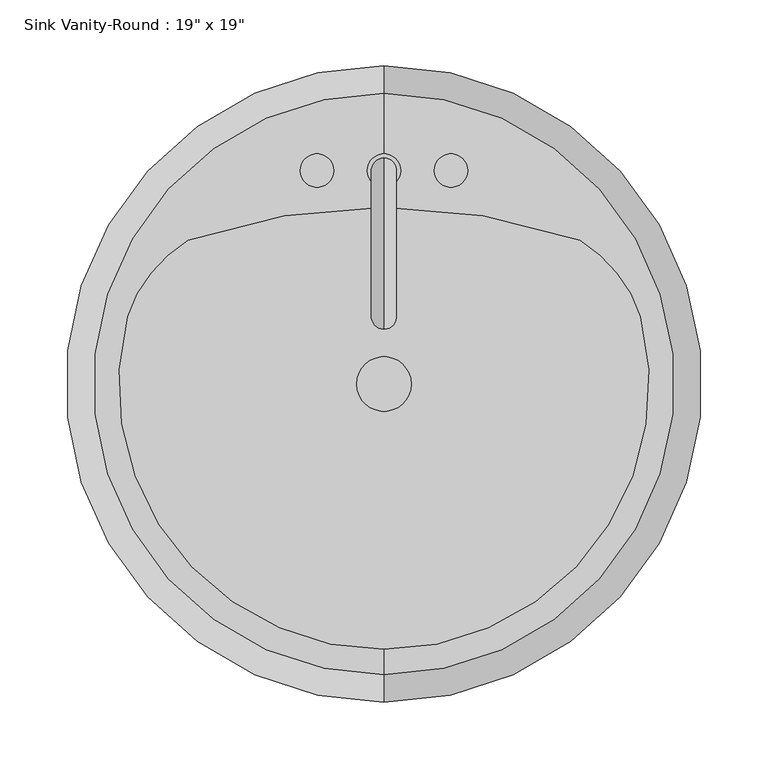
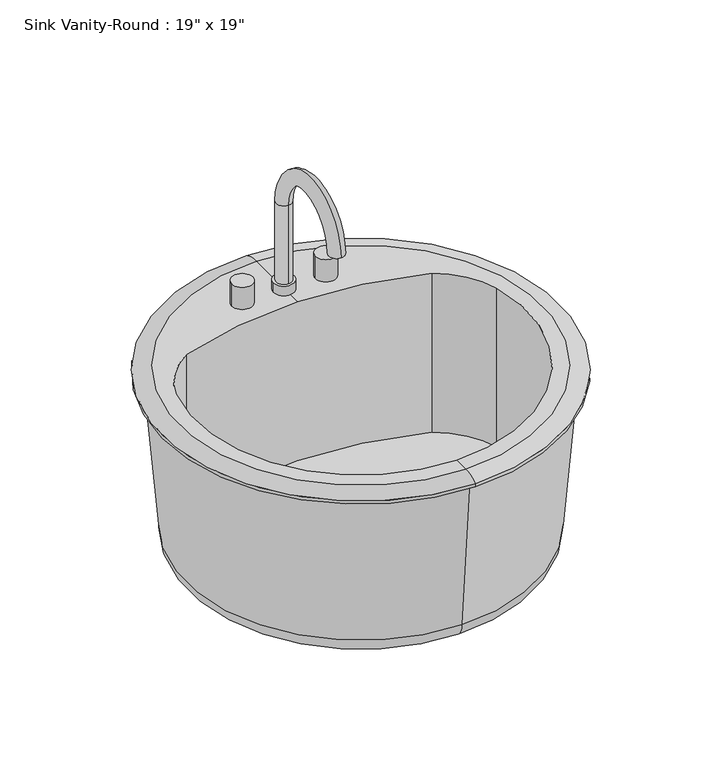
"""IFC4 building model written with IfcOpenShell, lengths in millimetres: flow terminal geometry."""

from ifc_helpers import new_model, si_unit, point, frame, frame_2d, origin, place, context, project, spatial, polyline, circle_curve, ellipse_curve, trimmed, segment, composite_curve, outline, extrude, source, transform, mapped, element, save
from ifc_brep_helpers import plane_surface, cylinder_surface, revolved_surface, advanced_brep


def flow_terminal_d49f872f(model_context):
    return source(origin(), model_context, "Body", "SolidModel", [
        advanced_brep(
        [(83.9517406, 247.0927185, 796.925), (109.3517406, 247.0927185, 796.925), (96.6517406, 237.5677185, 909.6375), (96.6517406, 256.6177185, 909.6375), (96.6517406, 256.6177185, 809.1602909), (96.6517406, 237.5677185, 809.1602909), (96.6517406, 145.7775038, 909.6375), (96.6517406, 126.7275038, 909.6375), (83.9517406, 247.0927185, 809.1602909), (109.3517406, 247.0927185, 809.1602909)],
        [
            (0, 1, circle_curve(frame((96.6517406, 247.0927185, 796.925), z_axis=(0.0, 0.0, -1.0), x_axis=(1.0, 0.0, 0.0)), 12.7)),
            (1, 0, circle_curve(frame((96.6517406, 247.0927185, 796.925), z_axis=(0.0, 0.0, -1.0), x_axis=(1.0, 0.0, 0.0)), 12.7)),
            (2, 3, circle_curve(frame((96.6517406, 247.0927185, 909.6375), z_axis=(0.0, 0.0, -1.0), x_axis=(0.0, 1.0, 0.0)), 9.525)),
            (3, 4),
            (4, 5, circle_curve(frame((96.6517406, 247.0927185, 809.1602909), z_axis=(0.0, 0.0, 1.0), x_axis=(0.0, 1.0, 0.0)), 9.525)),
            (5, 2),
            (3, 2, circle_curve(frame((96.6517406, 247.0927185, 909.6375), z_axis=(0.0, 0.0, -1.0), x_axis=(0.0, 1.0, 0.0)), 9.525)),
            (5, 4, circle_curve(frame((96.6517406, 247.0927185, 809.1602909), z_axis=(0.0, 0.0, 1.0), x_axis=(0.0, 1.0, 0.0)), 9.525)),
            (6, 7, circle_curve(frame((96.6517406, 136.2525038, 909.6375), z_axis=(0.0, 0.0, -1.0), x_axis=(0.0, -1.0, 0.0)), 9.525)),
            (7, 6, circle_curve(frame((96.6517406, 136.2525038, 909.6375), z_axis=(0.0, 0.0, -1.0), x_axis=(0.0, -1.0, 0.0)), 9.525)),
            (2, 6, circle_curve(frame((96.6517406, 191.6726112, 909.6375), z_axis=(1.0, 0.0, 0.0), x_axis=(0.0, 1.0, 0.0)), 45.8951073)),
            (7, 3, circle_curve(frame((96.6517406, 191.6726112, 909.6375), z_axis=(-1.0, 0.0, 0.0), x_axis=(0.0, 1.0, 0.0)), 64.9451073)),
            (8, 9, circle_curve(frame((96.6517406, 247.0927185, 809.1602909), z_axis=(0.0, 0.0, 1.0), x_axis=(1.0, 0.0, 0.0)), 12.7)),
            (9, 8, circle_curve(frame((96.6517406, 247.0927185, 809.1602909), z_axis=(0.0, 0.0, 1.0), x_axis=(1.0, 0.0, 0.0)), 12.7)),
            (8, 0),
            (1, 9),
        ],
        [
            plane_surface(frame((96.6517406, 237.5677185, 796.925), z_axis=(0.0, 0.0, -1.0), x_axis=(1.0, 0.0, 0.0))),
            cylinder_surface(frame((96.6517406, 247.0927185, 796.925), z_axis=(0.0, 0.0, -1.0), x_axis=(0.0, 1.0, 0.0)), 9.525),
            plane_surface(frame((96.6517406, 191.6726112, 909.6375), z_axis=(0.0, 0.0, -1.0), x_axis=(0.0, -1.0, 0.0))),
            revolved_surface(trimmed(ellipse_curve(frame((96.6517406, 247.0927185, 909.6375), z_axis=(0.0, 0.0, -1.0), x_axis=(0.0, 1.0, 0.0)), 9.525, 9.525), [point((96.6517406, 237.5677185, 909.6375))], [point((96.6517406, 256.6177185, 909.6375))], True, "CARTESIAN"), (96.6517406, 191.6726112, 909.6375), (1.0, 0.0, 0.0)),
            revolved_surface(trimmed(ellipse_curve(frame((96.6517406, 247.0927185, 909.6375), z_axis=(0.0, 0.0, -1.0), x_axis=(0.0, 1.0, 0.0)), 9.525, 9.525), [point((96.6517406, 256.6177185, 909.6375))], [point((96.6517406, 237.5677185, 909.6375))], True, "CARTESIAN"), (96.6517406, 191.6726112, 909.6375), (1.0, 0.0, 0.0)),
            plane_surface(frame((109.3517406, 247.0927185, 809.1602909), z_axis=(0.0, 0.0, 1.0), x_axis=(0.0, 1.0, 0.0))),
            cylinder_surface(frame((96.6517406, 247.0927185, 796.925), z_axis=(0.0, 0.0, 1.0), x_axis=(1.0, 0.0, 0.0)), 12.7),
        ],
        [
            (0, [[1, 2]]),
            (1, [[3, 4, 5, 6]]),
            (1, [[7, -6, 8, -4]]),
            (2, [[9, 10]]),
            (3, [[-3, 11, -10, 12]]),
            (4, [[-7, -12, -9, -11]]),
            (5, [[13, 14], [-5, -8]]),
            (6, [[-13, 15, -2, 16]]),
            (6, [[-14, -16, -1, -15]]),
        ],
    ),
        extrude(outline(composite_curve([segment(trimmed(circle_curve(frame_2d((45.8517406, 247.0927185)), 12.7), [point((33.1517406, 247.0927185))], [point((58.5517406, 247.0927185))], False, "CARTESIAN"), True, "CONTINUOUS"), segment(trimmed(circle_curve(frame_2d((45.8517406, 247.0927185)), 12.7), [point((58.5517406, 247.0927185))], [point((33.1517406, 247.0927185))], False, "CARTESIAN"), True, "CONTINUOUS")], self_intersect=False)), frame((0.0, 0.0, 796.925), z_axis=(0.0, 0.0, 1.0), x_axis=(1.0, 0.0, 0.0)), (0.0, 0.0, 1.0), 28.575),
        extrude(outline(composite_curve([segment(trimmed(circle_curve(frame_2d((147.4517406, 247.0927185)), 12.7), [point((134.7517406, 247.0927185))], [point((160.1517406, 247.0927185))], False, "CARTESIAN"), True, "CONTINUOUS"), segment(trimmed(circle_curve(frame_2d((147.4517406, 247.0927185)), 12.7), [point((160.1517406, 247.0927185))], [point((134.7517406, 247.0927185))], False, "CARTESIAN"), True, "CONTINUOUS")], self_intersect=False)), frame((0.0, 0.0, 796.925), z_axis=(0.0, 0.0, 1.0), x_axis=(1.0, 0.0, 0.0)), (0.0, 0.0, 1.0), 28.575),
        extrude(outline(composite_curve([segment(trimmed(circle_curve(frame_2d((96.6517406, 85.1677185)), 20.6375), [point((76.0142406, 85.1677185))], [point((117.2892406, 85.1677185))], False, "CARTESIAN"), True, "CONTINUOUS"), segment(trimmed(circle_curve(frame_2d((96.6517406, 85.1677185)), 20.6375), [point((117.2892406, 85.1677185))], [point((76.0142406, 85.1677185))], False, "CARTESIAN"), True, "CONTINUOUS")], self_intersect=False)), frame((0.0, 0.0, 571.5), z_axis=(0.0, 0.0, 1.0), x_axis=(1.0, 0.0, 0.0)), (0.0, 0.0, 1.0), 21.1842611),
        advanced_brep(
        [(96.6517406, -135.3870093, 796.925), (96.6517406, 305.7224463, 796.925), (96.6517406, 326.4677185, 791.36875), (96.6517406, -156.1322815, 791.36875), (96.6517406, -116.2405705, 796.925), (-98.1703414, 136.2525038, 796.925), (-52.1534933, 194.0861398, 796.925), (96.6517406, 219.2662048, 796.925), (245.4569744, 194.0861398, 796.925), (291.4738225, 136.2525038, 796.925), (96.6517406, -107.1264028, 571.5), (96.6517406, 277.4618398, 571.5), (96.6517406, 85.1677185, 571.5), (96.6517406, -127.6827361, 592.6842611), (96.6517406, 298.0181731, 592.6842611), (96.6517406, -144.2260315, 787.4), (96.6517406, 314.5614685, 787.4), (96.6517406, -156.1322815, 787.4), (96.6517406, 326.4677185, 787.4), (245.4569744, 194.0861398, 592.6842611), (-52.1534933, 194.0861398, 592.6842611), (-98.1703414, 136.2525038, 592.6842611), (291.4738225, 136.2525038, 592.6842611)],
        [
            (0, 1, circle_curve(frame((96.6517406, 85.1677185, 796.925), z_axis=(0.0, 0.0, -1.0), x_axis=(0.0, 1.0, 0.0)), 220.5547278)),
            (1, 2, circle_curve(frame((96.6517406, 309.4374616, 769.289434), z_axis=(-1.0, 0.0, 0.0), x_axis=(0.0, 1.0, 0.0)), 27.8841505)),
            (2, 3, circle_curve(frame((96.6517406, 85.1677185, 791.36875), z_axis=(0.0, 0.0, 1.0), x_axis=(0.0, 1.0, 0.0)), 241.3)),
            (3, 0, circle_curve(frame((96.6517406, -139.1020246, 769.289434), z_axis=(-1.0, 0.0, 0.0), x_axis=(0.0, -1.0, 0.0)), 27.8841505)),
            (1, 0, circle_curve(frame((96.6517406, 85.1677185, 796.925), z_axis=(0.0, 0.0, -1.0), x_axis=(0.0, 1.0, 0.0)), 220.5547278)),
            (3, 2, circle_curve(frame((96.6517406, 85.1677185, 791.36875), z_axis=(0.0, 0.0, 1.0), x_axis=(0.0, 1.0, 0.0)), 241.3)),
            (0, 4),
            (4, 5, circle_curve(frame((96.6517406, 85.1677185, 796.925), z_axis=(0.0, 0.0, -1.0), x_axis=(1.0, 0.0, 0.0)), 201.408289)),
            (5, 6, circle_curve(frame((1.3689689, 104.2755165, 796.925), z_axis=(0.0, 0.0, -1.0), x_axis=(1.0, 0.0, 0.0)), 104.5495194)),
            (6, 7, circle_curve(frame((96.6517406, -233.0168462, 796.925), z_axis=(0.0, 0.0, -1.0), x_axis=(1.0, 0.0, 0.0)), 452.283051)),
            (7, 1),
            (7, 8, circle_curve(frame((96.6517406, -233.0168462, 796.925), z_axis=(0.0, 0.0, -1.0), x_axis=(1.0, 0.0, 0.0)), 452.283051)),
            (8, 9, circle_curve(frame((191.9345122, 104.2755165, 796.925), z_axis=(0.0, 0.0, -1.0), x_axis=(1.0, 0.0, 0.0)), 104.5495194)),
            (9, 4, circle_curve(frame((96.6517406, 85.1677185, 796.925), z_axis=(0.0, 0.0, -1.0), x_axis=(1.0, 0.0, 0.0)), 201.408289)),
            (10, 11, circle_curve(frame((96.6517406, 85.1677185, 571.5), z_axis=(0.0, 0.0, -1.0), x_axis=(0.0, 1.0, 0.0)), 192.2941213)),
            (11, 12),
            (12, 10),
            (11, 10, circle_curve(frame((96.6517406, 85.1677185, 571.5), z_axis=(0.0, 0.0, -1.0), x_axis=(0.0, 1.0, 0.0)), 192.2941213)),
            (10, 13, circle_curve(frame((96.6517406, -107.1264028, 592.0656396), z_axis=(-1.0, 0.0, 0.0), x_axis=(0.0, -1.0, 0.0)), 20.5656396)),
            (13, 14, circle_curve(frame((96.6517406, 85.1677185, 592.6842611), z_axis=(0.0, 0.0, -1.0), x_axis=(0.0, 1.0, 0.0)), 212.8504546)),
            (14, 11, circle_curve(frame((96.6517406, 277.4618398, 592.0656396), z_axis=(-1.0, 0.0, 0.0), x_axis=(0.0, 1.0, 0.0)), 20.5656396)),
            (14, 13, circle_curve(frame((96.6517406, 85.1677185, 592.6842611), z_axis=(0.0, 0.0, -1.0), x_axis=(0.0, 1.0, 0.0)), 212.8504546)),
            (13, 15),
            (15, 16, circle_curve(frame((96.6517406, 85.1677185, 787.4), z_axis=(0.0, 0.0, -1.0), x_axis=(0.0, 1.0, 0.0)), 229.39375)),
            (16, 14),
            (16, 15, circle_curve(frame((96.6517406, 85.1677185, 787.4), z_axis=(0.0, 0.0, -1.0), x_axis=(0.0, 1.0, 0.0)), 229.39375)),
            (15, 17),
            (17, 18, circle_curve(frame((96.6517406, 85.1677185, 787.4), z_axis=(0.0, 0.0, -1.0), x_axis=(0.0, 1.0, 0.0)), 241.3)),
            (18, 16),
            (18, 17, circle_curve(frame((96.6517406, 85.1677185, 787.4), z_axis=(0.0, 0.0, -1.0), x_axis=(0.0, 1.0, 0.0)), 241.3)),
            (2, 18),
            (17, 3),
            (19, 20, circle_curve(frame((96.6517406, -233.0168462, 592.6842611), z_axis=(0.0, 0.0, 1.0), x_axis=(1.0, 0.0, 0.0)), 452.283051)),
            (20, 21, circle_curve(frame((1.3689689, 104.2755165, 592.6842611), z_axis=(0.0, 0.0, 1.0), x_axis=(1.0, 0.0, 0.0)), 104.5495194)),
            (21, 22, circle_curve(frame((96.6517406, 85.1677185, 592.6842611), z_axis=(0.0, 0.0, 1.0), x_axis=(1.0, 0.0, 0.0)), 201.408289)),
            (22, 19, circle_curve(frame((191.9345122, 104.2755165, 592.6842611), z_axis=(0.0, 0.0, 1.0), x_axis=(1.0, 0.0, 0.0)), 104.5495194)),
            (19, 8),
            (6, 20),
            (5, 21),
            (9, 22),
        ],
        [
            revolved_surface(trimmed(ellipse_curve(frame((96.6517406, 309.4374616, 769.289434), z_axis=(1.0, 0.0, 0.0), x_axis=(0.0, 1.0, 0.0)), 27.8841505, 27.8841505), [point((96.6517406, 326.4677185, 791.36875))], [point((96.6517406, 305.7224463, 796.925))], True, "CARTESIAN"), (96.6517406, 85.1677185, 796.925), (0.0, 0.0, 1.0)),
            plane_surface(frame((96.6517406, 85.1677185, 796.925), z_axis=(0.0, 0.0, 1.0), x_axis=(0.0, 1.0, 0.0))),
            plane_surface(frame((96.6517406, 85.1677185, 571.5), z_axis=(0.0, 0.0, -1.0), x_axis=(0.0, 1.0, 0.0))),
            revolved_surface(trimmed(ellipse_curve(frame((96.6517406, 277.4618398, 592.0656396), z_axis=(1.0, 0.0, 0.0), x_axis=(0.0, 1.0, 0.0)), 20.5656396, 20.5656396), [point((96.6517406, 277.4618398, 571.5))], [point((96.6517406, 298.0181731, 592.6842611))], True, "CARTESIAN"), (96.6517406, 85.1677185, 796.925), (0.0, 0.0, 1.0)),
            revolved_surface(polyline([(96.6517406, 298.0181731, 592.6842611), (96.6517406, 314.5614685, 787.4)]), (96.6517406, 85.1677185, 796.925), (0.0, 0.0, 1.0)),
            plane_surface(frame((96.6517406, 85.1677185, 787.4), z_axis=(0.0, 0.0, -1.0), x_axis=(0.0, 1.0, 0.0))),
            cylinder_surface(frame((96.6517406, 85.1677185, 796.925), z_axis=(0.0, 0.0, 1.0), x_axis=(0.0, 1.0, 0.0)), 241.3),
            plane_surface(frame((548.9347916, -233.0168462, 592.6842611), z_axis=(0.0, 0.0, 1.0), x_axis=(0.0, -1.0, 0.0))),
            revolved_surface(polyline([(548.9347916, -233.0168462, 796.925), (548.9347916, -233.0168462, 592.6842611)]), (96.6517406, -233.0168462, 592.6842611), (0.0, 0.0, 1.0)),
            revolved_surface(polyline([(105.91848829999999, 104.2755165, 796.925), (105.91848829999999, 104.2755165, 592.6842611)]), (1.3689689, 104.2755165, 592.6842611), (0.0, 0.0, 1.0)),
            revolved_surface(polyline([(298.0600296, 85.1677185, 796.925), (298.0600296, 85.1677185, 592.6842611)]), (96.6517406, 85.1677185, 592.6842611), (0.0, 0.0, 1.0)),
            revolved_surface(polyline([(296.4840316, 104.2755165, 796.925), (296.4840316, 104.2755165, 592.6842611)]), (191.9345122, 104.2755165, 592.6842611), (0.0, 0.0, 1.0)),
        ],
        [
            (0, [[1, 2, 3, 4]]),
            (0, [[-2, 5, -4, 6]]),
            (1, [[-1, 7, 8, 9, 10, 11]]),
            (1, [[-5, -11, 12, 13, 14, -7]]),
            (2, [[15, 16, 17]]),
            (2, [[-16, 18, -17]]),
            (3, [[-15, 19, 20, 21]]),
            (3, [[-18, -21, 22, -19]]),
            (4, [[-20, 23, 24, 25]]),
            (4, [[-22, -25, 26, -23]]),
            (5, [[-24, 27, 28, 29]]),
            (5, [[-26, -29, 30, -27]]),
            (6, [[-3, 31, -28, 32]]),
            (6, [[-6, -32, -30, -31]]),
            (7, [[33, 34, 35, 36]]),
            (8, [[-33, 37, -12, -10, 38]]),
            (9, [[-34, -38, -9, 39]]),
            (10, [[-35, -39, -8, -14, 40]]),
            (11, [[-36, -40, -13, -37]]),
        ],
    ),
    ])


if __name__ == "__main__":
    model = new_model("IFC4")
    model_context = context("Model", 3, world=origin())
    ifc_project = project(units=[si_unit("LENGTHUNIT", "METRE", prefix="MILLI")], contexts=[model_context])
    site = spatial("IfcSite", under=ifc_project)
    building = spatial("IfcBuilding", under=site)
    placement = place(None, origin())
    flow_terminal_shape = flow_terminal_d49f872f(model_context)
    element("IfcFlowTerminal", 1, ObjectType="Sink Vanity-Round : 19\" x 19\"", at=placement, inside=building, context=model_context, shape_type="MappedRepresentation", body=[
        mapped(flow_terminal_shape, transform((0.0, 0.0, 0.0), x_axis=(1.0, 0.0, 0.0), y_axis=(0.0, 1.0, 0.0), z_axis=(0.0, 0.0, 1.0))),
    ])
    save(model, "model.ifc")

# Revit data of these elements
# Type "Sink Vanity-Round : 19\" x 19\""
#   Assembly Code = "D2010400"
#   Top Of Counter = 2' - 7"
#   Basin Material = Porcelain, Linen
#   Faucet Material = Steel, Polished
#   Default Elevation = 0
# Element 1 (IfcFlowTerminal, "Sink Vanity-Round : 19\" x 19\"")
#   Materials on its faces: "Porcelain, Linen", "Steel, Polished"
# Materials
#   "Porcelain, Linen": class "Ceramic", colour RGB 249 239 230, transparency 0, Description = "Porcelain, linen", Cost = 0
#   "Steel, Polished": class "Metal", colour RGB 192 192 192, transparency 0, Description = "Polished steel", Cost = 0
